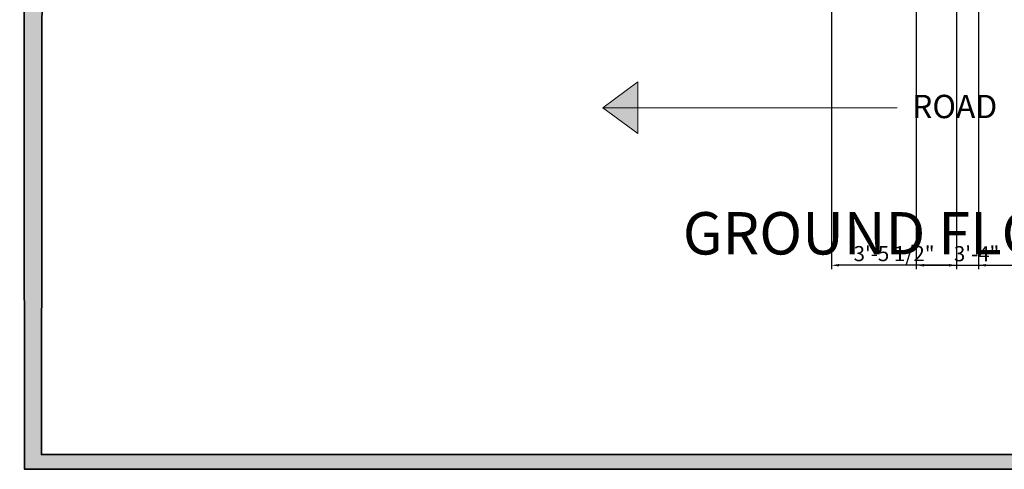
# Model space of a CAD drawing. Units: inches. Extents: x 1804 to 3296, y 909 to 2477.
# Tile 1 of 31: x 1804 to 2130, y 909 to 1059. Entities that reach past the tile are written whole.
import ezdxf

# ---------------------------------------------------------------- set-up
doc = ezdxf.new("R2010")
doc.units = ezdxf.units.IN
for name, color, linetype, lineweight in [('A-ANNO-DIMS', 2, 'Continuous', 18), ('A-ANNO-SYMB', 7, 'Continuous', 18), ('A-ANNO-TTLB', 156, 'Continuous', 35), ('A-WALL-PATT', 10, 'Continuous', 13), ('TEXT', 190, 'Continuous', 18)]:
    doc.layers.add(name, color=color, linetype=linetype, lineweight=lineweight)
doc.styles.get("Standard").update_dxf_attribs({"font": 'arial.ttf'})
doc.dimstyles.new('ISO-25', dxfattribs={"dimtxt": 5, "dimasz": 2.5, "dimexe": 1.25, "dimexo": 0.625, "dimtad": 1, "dimdec": 0, "dimlunit": 4, "dimtxsty": 'Standard', "dimcen": 2.5, "dimadec": 0, "dimazin": 0, "dimtfac": 1, "dimtdec": 0, "dimtmove": 0, "dimatfit": 3, "dimfxl": 1, "dimarcsym": 0})

# ---------------------------------------------------------------- blocks, each defined once
blk = doc.blocks.new('ROAD-DIRECTION')
h = blk.add_hatch(color=256)
h.dxf.hatch_style = 1
h.paths.add_polyline_path([(11.63, 8.56), (0, 8.56), (11.63, 0)])
h.paths.add_polyline_path([(11.63, 17.12), (0, 8.56), (11.63, 8.56)])
for p, q in [((0, 8.56), (11.63, 17.12)), ((11.63, 0), (11.63, 17.12)), ((97.65, 8.56), (0, 8.56)), ((0, 8.56), (11.63, 0))]:
    blk.add_line(p, q)
blk = doc.blocks.new('*D59')
at = {"layer": 'A-ANNO-DIMS', "color": 0, "lineweight": -2, "transparency": 16777216}
for p, q in [((2121.83, 1590.3), (2121.83, 975.89)), ((2161.83, 1590.3), (2161.83, 975.89)), ((2124.33, 977.14), (2159.33, 977.14))]:
    blk.add_line(p, q, dxfattribs=at)
at = {"layer": 'A-ANNO-DIMS', "color": 0, "lineweight": 100, "transparency": 16777216}
for points in [[(2124.33, 977.56), (2124.33, 976.72), (2121.83, 977.14)], [(2159.33, 977.56), (2159.33, 976.72), (2161.83, 977.14)]]:
    blk.add_solid(points, dxfattribs=at)
at = {"layer": 'Defpoints', "color": 0, "lineweight": 100, "transparency": 16777216}
for p in [(2121.83, 1590.92), (2161.83, 1590.92), (2161.83, 977.14)]:
    blk.add_point(p, dxfattribs=at)
at = {"layer": 'A-ANNO-DIMS', "color": 0, "transparency": 16777216, "insert": (2141.83, 980.32), "char_height": 5, "attachment_point": 5}
blk.add_mtext('3\'-4"', dxfattribs=at)
blk = doc.blocks.new('*D60')
at = {"layer": 'A-ANNO-DIMS', "color": 0, "lineweight": -2, "transparency": 16777216}
for p, q in [((2073.08, 1544.95), (2073.08, 975.89)), ((2114.58, 1543.75), (2114.58, 975.89)), ((2112.08, 977.14), (2075.58, 977.14))]:
    blk.add_line(p, q, dxfattribs=at)
at = {"layer": 'A-ANNO-DIMS', "color": 0, "lineweight": 100, "transparency": 16777216}
for points in [[(2075.58, 977.56), (2075.58, 976.72), (2073.08, 977.14)], [(2112.08, 977.56), (2112.08, 976.72), (2114.58, 977.14)]]:
    blk.add_solid(points, dxfattribs=at)
at = {"layer": 'Defpoints', "color": 0, "lineweight": 100, "transparency": 16777216}
for p in [(2073.08, 1545.58), (2114.58, 1544.38), (2073.08, 977.14)]:
    blk.add_point(p, dxfattribs=at)
at = {"layer": 'A-ANNO-DIMS', "color": 0, "transparency": 16777216, "insert": (2093.83, 980.35), "char_height": 5, "attachment_point": 5}
blk.add_mtext('3\'-5 1/2"', dxfattribs=at)
blk = doc.blocks.new('*D61')
at = {"layer": 'A-ANNO-DIMS', "color": 0, "lineweight": -2, "transparency": 16777216}
for p, q in [((2101.21, 1137.44), (2101.21, 975.89)), ((2141.21, 1137.44), (2141.21, 975.89)), ((2103.71, 977.14), (2138.71, 977.14))]:
    blk.add_line(p, q, dxfattribs=at)
at = {"layer": 'A-ANNO-DIMS', "color": 0, "lineweight": 100, "transparency": 16777216}
for points in [[(2103.71, 977.56), (2103.71, 976.72), (2101.21, 977.14)], [(2138.71, 977.56), (2138.71, 976.72), (2141.21, 977.14)]]:
    blk.add_solid(points, dxfattribs=at)
at = {"layer": 'Defpoints', "color": 0, "lineweight": 100, "transparency": 16777216}
for p in [(2101.21, 1138.07), (2141.21, 1138.07), (2141.21, 977.14)]:
    blk.add_point(p, dxfattribs=at)
at = {"layer": 'A-ANNO-DIMS', "color": 0, "transparency": 16777216, "insert": (2121.21, 980.32), "char_height": 5, "attachment_point": 5}
blk.add_mtext('3\'-4"', dxfattribs=at)

msp = doc.modelspace()

# ---------------------------------------------------------------- hatches: boundary and pattern name
at = {"layer": 'A-ANNO-TTLB'}
h = msp.add_hatch(color=256, dxfattribs=at)
h.dxf.hatch_style = 1
h.paths.add_polyline_path([(3294.53, 2476.54), (1803.79, 2476.54), (1805.43, 909.47), (3296.17, 909.47)])
h.paths.add_polyline_path([(1811, 914.33), (1812.79, 2467.54), (3285.53, 2467.54), (3283.74, 914.33)], flags=16)
h.paths.add_polyline_path([(1925.58, 1062.77), (1925.58, 1138.07), (1925.58, 1539.88), (1925.58, 1793.38), (1925.58, 1830.04), (2325.54, 1830.04), (2325.54, 1793.38), (2325.54, 1586.42), (2325.54, 1138.07), (2325.54, 1062.77)], flags=0)
h.paths.add_polyline_path([(1997.22, 1029.4), (2008.85, 1037.96), (2008.85, 1020.84)], flags=0)
h.paths.add_polyline_path([(1934.58, 1138.07), (1934.58, 1147.07), (2078.77, 1147.07), (2078.77, 1138.07), (2060.94, 1138.07)], flags=0)
h.paths.add_polyline_path([(1944.35, 1138.07), (1944.35, 1147.07), (2056.05, 1147.07), (2056.05, 1138.07)], flags=0)
h.paths.add_polyline_path([(2222.24, 1037.96), (2233.87, 1029.4), (2222.24, 1020.84)], flags=0)
h.paths.add_polyline_path([(2061.94, 1139.07), (2061.94, 1146.07), (2077.77, 1146.07), (2077.77, 1139.07)], flags=0)
h.paths.add_polyline_path([(2149.58, 1138.07), (2149.58, 1269.44), (2158.58, 1269.44), (2158.58, 1326.69), (2149.58, 1326.69), (2149.58, 1340.94), (2139.6, 1340.94), (2139.6, 1434.25), (2149.58, 1434.25), (2149.58, 1447.36), (2158.58, 1447.36), (2158.58, 1423.87), (2158.58, 1408.06), (2198.46, 1408.06), (2198.46, 1412.56), (2282.65, 1412.56), (2282.65, 1465.94), (2316.54, 1465.94), (2316.54, 1590.92), (2192.86, 1590.92), (2192.86, 1595.3), (2291.17, 1595.3), (2291.17, 1590.92), (2316.54, 1590.92), (2316.54, 1784.38), (2300.24, 1784.38), (2300.24, 1757.47), (2268, 1757.47), (2268, 1681.04), (2180.87, 1681.04), (2180.87, 1757.47), (2148.63, 1757.47), (2148.63, 1784.38), (2119.08, 1784.38), (2119.08, 1585.58), (2114.58, 1585.58), (2114.58, 1784.38), (2064.11, 1784.38), (2046.28, 1784.38), (2046.28, 1760.38), (1958.58, 1760.38), (1958.58, 1664.38), (1934.58, 1664.38), (1934.58, 1784.38), (1934.58, 1793.38), (2046.28, 1793.38), (2064.11, 1793.38), (2119.08, 1793.38), (2230.78, 1793.38), (2230.78, 1784.38), (2268, 1784.38), (2300.24, 1784.38), (2316.54, 1784.38), (2316.54, 1590.92), (2316.54, 1373.73), (2316.54, 1138.07)], flags=0)
h.paths.add_polyline_path([(2209.19, 1166.63), (2209.19, 1175.63), (2158.58, 1175.63), (2209.19, 1223.63), (2209.19, 1231.63), (2183.88, 1231.63), (2183.88, 1301.66), (2242.59, 1301.66), (2242.59, 1326.69), (2316.54, 1326.69), (2272.59, 1271.63), (2272.59, 1223.63), (2316.54, 1175.63), (2272.59, 1175.63), (2272.59, 1166.63)], flags=0)
h.paths.add_polyline_path([(1947.77, 1345.22), (1947.77, 1457.48), (1991.2, 1457.48), (1991.2, 1451.7), (1991.2, 1352.18), (1991.2, 1345.22)], flags=0)
h.paths.add_polyline_path([(2209.19, 1271.63), (2262.59, 1271.63), (2262.59, 1311.85), (2272.59, 1301.66), (2272.59, 1271.63), (2269.92, 1269.63), (2270.59, 1269.63), (2270.59, 1225.63), (2211.19, 1225.63), (2211.19, 1269.63), (2211.86, 1269.63)], flags=0)
h.paths.add_polyline_path([(2000.34, 1378.21), (2000.34, 1429.71), (2025.22, 1429.71), (2025.22, 1378.21)], flags=0)
h.paths.add_polyline_path([(2001.34, 1379.21), (2001.34, 1428.71), (2024.22, 1428.71), (2024.22, 1379.21)], flags=0)
h.paths.add_polyline_path([(2012.34, 1390.21), (2012.34, 1417.71), (2013.22, 1417.71), (2013.22, 1390.21)], flags=0)
h.paths.add_polyline_path([(2237.56, 1331.19), (2237.56, 1340.18), (2238.62, 1340.18), (2238.62, 1386.84), (2241.04, 1386.84), (2242.06, 1386.84), (2242.06, 1408.06), (2316.54, 1331.19)], flags=0)
h.paths.add_polyline_path([(1953.73, 1464.35), (1953.73, 1498.59), (1981.74, 1498.59), (1981.74, 1464.35)], flags=0)
h.paths.add_polyline_path([(1987.63, 1462.08), (1987.63, 1500.95), (2104.07, 1500.95), (2104.07, 1462.08), (2099.27, 1462.08), (1993.6, 1462.08)], flags=0)
h.paths.add_polyline_path([(1956.06, 1481.47, -1), (1979.41, 1481.47, -1)], flags=0)
edge = h.paths.add_edge_path(flags=0)
edge.add_ellipse((2299.53, 1438.37), major_axis=(0.31, 21.36), ratio=0.670333, start_angle=0, end_angle=360)
h.paths.add_polyline_path([(2297.39, 1438.37, -1), (2301.67, 1438.37, -1)], flags=0)
h.paths.add_polyline_path([(2591.54, 1163.23), (2591.54, 1179.38), (2591.54, 1379.68), (2591.54, 1395.84), (2734.5, 1395.84), (2734.5, 1379.68), (2734.5, 1179.38), (2734.5, 1163.23)], flags=0)
h.paths.add_polyline_path([(2592.54, 1164.23), (2592.54, 1166.23), (2733.5, 1166.23), (2733.5, 1164.23)], flags=0)
h.paths.add_polyline_path([(2592.54, 1180.38), (2592.54, 1378.68), (2733.5, 1378.68), (2733.5, 1180.38)], flags=0)
h.paths.add_polyline_path([(2593.54, 1181.38), (2593.54, 1377.68), (2732.5, 1377.68), (2732.5, 1181.38)], flags=0)
h.paths.add_polyline_path([(2594.54, 1182.38), (2594.54, 1376.68), (2731.5, 1376.68), (2731.5, 1182.38)], flags=0)
h.paths.add_polyline_path([(1936.95, 1697.46), (1936.95, 1736.46), (1955.41, 1736.46), (1955.41, 1697.46)], flags=0)
h.paths.add_polyline_path([(1938.48, 1718.36), (1938.48, 1734.92), (1953.65, 1734.92), (1953.65, 1718.36)], flags=0)
h.paths.add_polyline_path([(1944.75, 1726.64, -1), (1947.37, 1726.64, -1)], flags=0)
h.paths.add_polyline_path([(2592.54, 1394.84), (2733.5, 1394.84), (2733.5, 1392.84), (2592.54, 1392.84)], flags=0)
h.paths.add_polyline_path([(1976.61, 1762.5), (1976.61, 1781.44), (2012.79, 1781.44), (2012.79, 1762.5)], flags=0)
h.paths.add_polyline_path([(1979.57, 1771.97, -1), (1991.39, 1771.97, -1)], flags=0)
h.paths.add_polyline_path([(1995.36, 1771.97, -1), (2007.18, 1771.97, -1)], flags=0)
h.paths.add_polyline_path([(2251.51, 1744.53), (2268, 1730.05), (2251.51, 1730.05)], flags=0)
h.paths.add_polyline_path([(2047.28, 1785.38), (2047.28, 1792.38), (2063.11, 1792.38), (2063.11, 1785.38)], flags=0)
h.paths.add_polyline_path([(2155.08, 1770.92, -1), (2174.42, 1770.92, -1)], flags=0)
h.paths.add_polyline_path([(2188.59, 1758.27), (2188.59, 1772.81), (2222.3, 1772.81), (2222.3, 1758.27)], flags=0)
h.paths.add_polyline_path([(2223.97, 1758.27), (2223.97, 1772.81), (2257.68, 1772.81), (2257.68, 1758.27)], flags=0)
h.paths.add_polyline_path([(2274.45, 1770.92, -1), (2293.8, 1770.92, -1)], flags=0)
h.paths.add_polyline_path([(2591.54, 1582.09), (2591.54, 1782.39), (2734.5, 1782.39), (2734.5, 1582.09)], flags=0)
h.paths.add_polyline_path([(2592.54, 1583.09), (2592.54, 1781.39), (2733.5, 1781.39), (2733.5, 1583.09)], flags=0)
h.paths.add_polyline_path([(2593.54, 1584.09), (2593.54, 1780.39), (2732.5, 1780.39), (2732.5, 1584.09)], flags=0)
h.paths.add_polyline_path([(2594.54, 1585.09), (2594.54, 1779.39), (2731.5, 1779.39), (2731.5, 1585.09)], flags=0)
h.paths.add_polyline_path([(1922.17, 1978.79), (1922.17, 2295.08), (1922.17, 2296.08), (2115.67, 2296.08), (2115.67, 2384.31), (2115.67, 2385.31), (2322.12, 2385.31), (2323.12, 2385.31), (2323.12, 1979.79), (2323.12, 1978.79), (1923.17, 1978.79)], flags=0)
h.paths.add_polyline_path([(1922.17, 1978.79), (1922.17, 2051.31), (1922.17, 2214.86), (1922.17, 2296.08), (2115.67, 2296.08), (2115.67, 2385.31), (2323.12, 2385.31), (2323.12, 2280.42), (2323.12, 1978.79), (2115.67, 1978.79)], flags=0)
h.paths.add_polyline_path([(1923.17, 1979.79), (1923.17, 2050.31), (2115.67, 2050.31), (2115.67, 2051.31), (1923.17, 2051.31), (1923.17, 2213.86), (1923.17, 2214.86), (1923.17, 2295.08), (1990.02, 2295.08), (1990.02, 2214.86), (1991.02, 2214.86), (1991.02, 2295.08), (2115.67, 2295.08), (2115.67, 1979.79), (2116.67, 1979.79), (2116.67, 2304.18), (2116.67, 2384.31), (2322.12, 2384.31), (2322.12, 2280.42), (2322.12, 1979.79), (2115.67, 1979.79)], flags=0)
h.paths.add_polyline_path([(2972.46, 1192.5), (2972.46, 1196.92), (2995.47, 1196.92), (2995.47, 1255.47), (2995.09, 1255.47), (2987.42, 1249.39), (2980.08, 1255.47), (2978.05, 1255.47), (2978.05, 1257.24), (2995.47, 1257.24), (2995.47, 1261.58), (3015.37, 1261.58), (3015.37, 1333.28), (3015.37, 1414.4), (3032.82, 1414.4), (3032.82, 1333.28), (3032.82, 1261.58), (3052.66, 1261.58), (3052.66, 1255.47), (3079.86, 1255.47), (3078.72, 1254.57), (3081.47, 1252.29), (3078.56, 1249.99), (3075.81, 1252.26), (3072.57, 1249.69), (3070.36, 1251.52), (3067.67, 1249.39), (3060.34, 1255.47), (3052.66, 1255.47), (3052.66, 1196.92), (3054.58, 1196.92), (3074, 1196.92), (3074, 1192.5), (3052.66, 1192.5), (2995.47, 1192.5)], flags=0)
h.paths.add_polyline_path([(2490.75, 1979.27), (2490.75, 1980.27), (2596.87, 1980.27), (2596.87, 2051.8), (2596.87, 2052.8), (2596.87, 2216.35), (2596.87, 2297.57), (2717.32, 2297.57), (2710.57, 2305.62), (2724.07, 2305.62), (2717.32, 2297.57), (2782.37, 2297.57), (2782.37, 2395.8), (3006.82, 2395.8), (3006.82, 1981.27), (3093.73, 1981.27), (3093.73, 1980.27), (3047.51, 1980.27), (3046.37, 1979.37), (3049.11, 1977.1), (3046.2, 1974.79), (3043.46, 1977.07), (3040.21, 1974.49), (3038, 1976.32), (3035.32, 1974.2), (3027.98, 1980.27), (2871.83, 1980.27), (2871.83, 1981.27), (2791.37, 1981.27), (2791.37, 2050.8), (2597.87, 2050.8), (2597.87, 1980.27), (2597.87, 1979.27), (2546.27, 1979.27), (2545.12, 1978.37), (2547.87, 1976.1), (2544.96, 1973.79), (2542.22, 1976.07), (2538.97, 1973.49), (2536.76, 1975.32), (2534.07, 1973.2), (2526.74, 1979.27)], flags=0)
h.paths.add_polyline_path([(2597.87, 2051.8), (2606.87, 2051.8), (2606.87, 2258.39), (2597.87, 2258.39), (2597.87, 2296.57), (2606.87, 2296.57), (2606.87, 2262.39), (2782.37, 2262.39), (2782.37, 2296.57), (2790.37, 2296.57), (2790.37, 2262.39), (2791.37, 2262.39), (2791.37, 2305.67), (2791.37, 2385.8), (2996.82, 2385.8), (2996.82, 2339.85), (3006.82, 2339.85), (3006.82, 2250.12), (2997.82, 2250.12), (2997.82, 1981.27), (2996.82, 1981.27), (2872.83, 1981.27), (2872.83, 1991.8), (2871.83, 1991.8), (2871.83, 2050.8), (2790.37, 2050.8), (2597.87, 2050.8)], flags=0)
h.paths.add_polyline_path([(2179.93, 2153.92), (2179.93, 2353.97), (2259.98, 2353.97), (2259.98, 2153.92)], flags=0)
h.paths.add_polyline_path([(2180.93, 2154.92), (2180.93, 2352.97), (2258.98, 2352.97), (2258.98, 2154.92)], flags=0)
h.paths.add_polyline_path([(2960.87, 1608.49), (2960.87, 1753.62), (3070.9, 1753.62), (3070.9, 1608.49)], flags=0)
h.paths.add_polyline_path([(2961.87, 1609.49), (2961.87, 1752.62), (3069.9, 1752.62), (3069.9, 1609.49)], flags=0)
h.paths.add_polyline_path([(2962.87, 1610.49), (2962.87, 1751.62), (3068.9, 1751.62), (3068.9, 1610.49)], flags=0)
h.paths.add_polyline_path([(2963.87, 1611.49), (2963.87, 1750.62), (3067.9, 1750.62), (3067.9, 1611.49)], flags=0)
h.paths.add_polyline_path([(2782.37, 2051.8), (2782.37, 2216.32), (2791.37, 2216.32), (2791.37, 2051.8), (2872.83, 2051.8), (2872.83, 2068.56), (2884.67, 2068.56), (2884.67, 2085.33), (2896.51, 2085.33), (2896.51, 2102.09), (2908.36, 2102.09), (2908.36, 2118.85), (2920.2, 2118.85), (2920.2, 2135.62), (2932.05, 2135.62), (2932.05, 2145.3), (2925.08, 2145.3), (2925.08, 2203.2), (2996.82, 2203.2), (2996.82, 2145.3), (2953.82, 2145.3), (2872.83, 2051.8), (2790.37, 2051.8)], flags=0)
h.paths.add_polyline_path([(2717.32, 2238.65), (2710.57, 2246.7), (2724.07, 2246.7)], flags=0)
h.paths.add_polyline_path([(2003.09, 1122.79), (2017.16, 1122.79), (2017.16, 1138.74), (2003.09, 1138.74)], flags=8)
h.paths.add_polyline_path([(2174.76, 1792.72), (2188.83, 1792.72), (2188.83, 1808.66), (2174.76, 1808.66)], flags=8)
h.paths.add_polyline_path([(1987.95, 1792.51), (2002.02, 1792.51), (2002.02, 1808.45), (1987.95, 1808.45)], flags=8)
h.paths.add_polyline_path([(2148.79, 1289.26), (2160.46, 1289.26), (2160.46, 1305.2), (2148.79, 1305.2)], flags=8)
h.paths.add_polyline_path([(2115.36, 1133.57), (2127.04, 1133.57), (2127.04, 1149.51), (2115.36, 1149.51)], flags=8)
h.paths.add_polyline_path([(2237.58, 1421.48), (2249.25, 1421.48), (2249.25, 1437.43), (2237.58, 1437.43)], flags=8)
h.paths.add_polyline_path([(2134.99, 1584.32), (2146.66, 1584.32), (2146.66, 1600.26), (2134.99, 1600.26)], flags=8)
h.paths.add_polyline_path([(2101.95, 1557.31), (2113.62, 1557.31), (2113.62, 1573.25), (2101.95, 1573.25)], flags=8)
h.paths.add_polyline_path([(2937.85, 1156.77), (3120.41, 1156.77), (3120.41, 1185.72), (2937.85, 1185.72)], flags=8)
h.paths.add_polyline_path([(2980.71, 1786.71), (3050.06, 1786.71), (3050.06, 1802.66), (2980.71, 1802.66)], flags=8)
h.paths.add_polyline_path([(2869.28, 1661.96), (2938.62, 1661.96), (2938.62, 1690.8), (2869.28, 1690.8)], flags=8)
h.paths.add_polyline_path([(3092.27, 1674.86), (3161.62, 1674.86), (3161.62, 1690.8), (3092.27, 1690.8)], flags=8)
h.paths.add_polyline_path([(2980.71, 1674.86), (3050.06, 1674.86), (3050.06, 1690.8), (2980.71, 1690.8)], flags=8)
h.paths.add_polyline_path([(2649.07, 1678.23), (2674.53, 1678.23), (2674.53, 1714.76), (2649.07, 1714.76)], flags=8)
h.paths.add_polyline_path([(2530.84, 1981.63), (2549.13, 1981.63), (2549.13, 1997.57), (2530.84, 1997.57)], flags=8)
h.paths.add_polyline_path([(3031.29, 1981.77), (3049.58, 1981.77), (3049.58, 1997.71), (3031.29, 1997.71)], flags=8)
h.paths.add_polyline_path([(2715.38, 1911.9), (2851.54, 1911.9), (2851.54, 1940.85), (2715.38, 1940.85)], flags=8)
h.paths.add_polyline_path([(2015.23, 1927.36), (2205.42, 1927.36), (2205.42, 1956.3), (2015.23, 1956.3)], flags=8)
h.paths.add_polyline_path([(2671.84, 2057.84), (2702.75, 2057.84), (2702.75, 2073.79), (2671.84, 2073.79)], flags=8)
h.paths.add_polyline_path([(2678.5, 2316.52), (2765.26, 2316.52), (2765.26, 2332.46), (2678.5, 2332.46)], flags=8)
h.paths.add_polyline_path([(2678.48, 2271.96), (2736.41, 2271.96), (2736.41, 2287.9), (2678.48, 2287.9)], flags=8)
h.paths.add_polyline_path([(2019.2, 972.79), (2243.21, 972.79), (2243.21, 1001.74), (2019.2, 1001.74)], flags=8)
h.paths.add_polyline_path([(2097.06, 1021.56), (2132.16, 1021.56), (2132.16, 1037.51), (2097.06, 1037.51)], flags=8)
h.paths.add_polyline_path([(2182.47, 1360.48), (2207.35, 1360.48), (2207.35, 1376.42), (2182.47, 1376.42)], flags=8)
h.paths.add_polyline_path([(2261.12, 1361.77), (2295.01, 1361.77), (2295.01, 1377.71), (2261.12, 1377.71)], flags=8)
h.paths.add_polyline_path([(2245.75, 1511.51), (2278.44, 1511.51), (2278.44, 1527.46), (2245.75, 1527.46)], flags=8)
h.paths.add_polyline_path([(1991.16, 1296.29), (2060.51, 1296.29), (2060.51, 1312.23), (1991.16, 1312.23)], flags=8)
h.paths.add_polyline_path([(2187, 1651.35), (2246.71, 1651.35), (2246.71, 1667.29), (2187, 1667.29)], flags=8)
h.paths.add_polyline_path([(1976.49, 1684.81), (2068.63, 1684.81), (2068.63, 1700.76), (1976.49, 1700.76)], flags=8)
at = {"layer": 'A-WALL-PATT'}
h = msp.add_hatch(color=256, dxfattribs=at)
h.dxf.hatch_style = 1
h.paths.add_polyline_path([(2119.08, 1544.38), (1925.58, 1544.38), (1925.58, 1539.88), (2119.08, 1539.88)])
h.paths.add_polyline_path([(2119.08, 1545.58), (2114.58, 1545.58), (2114.58, 1544.38), (2119.08, 1544.38)])
h.paths.add_polyline_path([(1965.87, 1658.79), (1965.87, 1679.09), (1955.57, 1679.09), (1955.57, 1658.79)], flags=9)
h.paths.add_polyline_path([(2293.18, 1677.29), (2293.18, 1697.58), (2282.88, 1697.58), (2282.88, 1677.29)], flags=9)
h.paths.add_polyline_path([(2271.13, 1545.23), (2287.53, 1545.23), (2287.53, 1555.53), (2271.13, 1555.53)], flags=9)
h.paths.add_polyline_path([(2303.26, 1488.52), (2303.26, 1508.82), (2292.95, 1508.82), (2292.95, 1488.52)], flags=9)
h.paths.add_polyline_path([(2271.13, 1393.15), (2287.53, 1393.15), (2287.53, 1403.45), (2271.13, 1403.45)], flags=9)
h.paths.add_polyline_path([(2306.48, 1361.45), (2306.48, 1377.86), (2296.18, 1377.86), (2296.18, 1361.45)], flags=9)
h.paths.add_polyline_path([(2174.54, 1361.45), (2174.54, 1377.86), (2164.23, 1377.86), (2164.23, 1361.45)], flags=9)
h.paths.add_polyline_path([(1968.21, 1333.34), (1968.21, 1353.64), (1957.91, 1353.64), (1957.91, 1333.34)], flags=9)
h.paths.add_polyline_path([(2003.09, 1122.79), (2017.16, 1122.79), (2017.16, 1138.74), (2003.09, 1138.74)], flags=9)
h.paths.add_polyline_path([(2174.76, 1792.72), (2188.83, 1792.72), (2188.83, 1808.66), (2174.76, 1808.66)], flags=9)
h.paths.add_polyline_path([(1987.95, 1792.51), (2002.02, 1792.51), (2002.02, 1808.45), (1987.95, 1808.45)], flags=9)
h.paths.add_polyline_path([(2148.79, 1289.26), (2160.46, 1289.26), (2160.46, 1305.2), (2148.79, 1305.2)], flags=9)
h.paths.add_polyline_path([(2115.36, 1133.57), (2127.04, 1133.57), (2127.04, 1149.51), (2115.36, 1149.51)], flags=9)
h.paths.add_polyline_path([(2237.58, 1421.48), (2249.25, 1421.48), (2249.25, 1437.43), (2237.58, 1437.43)], flags=9)
h.paths.add_polyline_path([(2134.99, 1584.32), (2146.66, 1584.32), (2146.66, 1600.26), (2134.99, 1600.26)], flags=9)
h.paths.add_polyline_path([(2101.95, 1557.31), (2113.62, 1557.31), (2113.62, 1573.25), (2101.95, 1573.25)], flags=9)
h.paths.add_polyline_path([(2937.85, 1156.77), (3120.41, 1156.77), (3120.41, 1185.72), (2937.85, 1185.72)], flags=9)
h.paths.add_polyline_path([(2980.71, 1786.71), (3050.06, 1786.71), (3050.06, 1802.66), (2980.71, 1802.66)], flags=9)
h.paths.add_polyline_path([(2869.28, 1661.96), (2938.62, 1661.96), (2938.62, 1690.8), (2869.28, 1690.8)], flags=9)
h.paths.add_polyline_path([(3092.27, 1674.86), (3161.62, 1674.86), (3161.62, 1690.8), (3092.27, 1690.8)], flags=9)
h.paths.add_polyline_path([(2980.71, 1674.86), (3050.06, 1674.86), (3050.06, 1690.8), (2980.71, 1690.8)], flags=9)
h.paths.add_polyline_path([(2649.07, 1678.23), (2674.53, 1678.23), (2674.53, 1714.76), (2649.07, 1714.76)], flags=9)
h.paths.add_polyline_path([(2530.84, 1981.63), (2549.13, 1981.63), (2549.13, 1997.57), (2530.84, 1997.57)], flags=9)
h.paths.add_polyline_path([(3031.29, 1981.77), (3049.58, 1981.77), (3049.58, 1997.71), (3031.29, 1997.71)], flags=9)
h.paths.add_polyline_path([(2715.38, 1911.9), (2851.54, 1911.9), (2851.54, 1940.85), (2715.38, 1940.85)], flags=9)
h.paths.add_polyline_path([(2015.23, 1927.36), (2205.42, 1927.36), (2205.42, 1956.3), (2015.23, 1956.3)], flags=9)
h.paths.add_polyline_path([(2671.84, 2057.84), (2702.75, 2057.84), (2702.75, 2073.79), (2671.84, 2073.79)], flags=9)
h.paths.add_polyline_path([(2678.5, 2316.52), (2765.26, 2316.52), (2765.26, 2332.46), (2678.5, 2332.46)], flags=9)
h.paths.add_polyline_path([(2678.48, 2271.96), (2736.41, 2271.96), (2736.41, 2287.9), (2678.48, 2287.9)], flags=9)
h.paths.add_polyline_path([(2019.2, 972.79), (2243.21, 972.79), (2243.21, 1001.74), (2019.2, 1001.74)], flags=9)
h.paths.add_polyline_path([(2097.06, 1021.56), (2132.16, 1021.56), (2132.16, 1037.51), (2097.06, 1037.51)], flags=9)
h.paths.add_polyline_path([(2182.47, 1360.48), (2207.35, 1360.48), (2207.35, 1376.42), (2182.47, 1376.42)], flags=9)
h.paths.add_polyline_path([(2261.12, 1361.77), (2295.01, 1361.77), (2295.01, 1377.71), (2261.12, 1377.71)], flags=9)
h.paths.add_polyline_path([(2245.75, 1511.51), (2278.44, 1511.51), (2278.44, 1527.46), (2245.75, 1527.46)], flags=9)
h.paths.add_polyline_path([(1991.16, 1296.29), (2060.51, 1296.29), (2060.51, 1312.23), (1991.16, 1312.23)], flags=9)
h.paths.add_polyline_path([(2187, 1651.35), (2246.71, 1651.35), (2246.71, 1667.29), (2187, 1667.29)], flags=9)
h.paths.add_polyline_path([(1976.49, 1684.81), (2068.63, 1684.81), (2068.63, 1700.76), (1976.49, 1700.76)], flags=9)
h = msp.add_hatch(color=256, dxfattribs=at)
h.dxf.hatch_style = 1
h.paths.add_polyline_path([(2149.58, 1147.07), (2141.21, 1147.07), (2141.21, 1144.07), (2141.21, 1138.07), (2149.58, 1138.07)])
h.paths.add_polyline_path([(2101.21, 1144.07, -0.01877), (2101.32, 1147.07), (2078.77, 1147.07), (2078.77, 1138.07), (2101.21, 1138.07)])
h.paths.add_polyline_path([(2060.94, 1147.07), (2056.05, 1147.07), (2056.05, 1138.07), (2060.94, 1138.07)])
h.paths.add_polyline_path([(1944.35, 1147.07), (1934.58, 1147.07), (1934.58, 1138.07), (1944.35, 1138.07)])
h.paths.add_polyline_path([(2158.58, 1269.44), (2149.58, 1269.44), (2149.58, 1138.07), (2158.58, 1138.07)])
h.paths.add_polyline_path([(2003.09, 1122.79), (2017.16, 1122.79), (2017.16, 1138.74), (2003.09, 1138.74)], flags=9)
h.paths.add_polyline_path([(2174.76, 1792.72), (2188.83, 1792.72), (2188.83, 1808.66), (2174.76, 1808.66)], flags=9)
h.paths.add_polyline_path([(1987.95, 1792.51), (2002.02, 1792.51), (2002.02, 1808.45), (1987.95, 1808.45)], flags=9)
h.paths.add_polyline_path([(2148.79, 1289.26), (2160.46, 1289.26), (2160.46, 1305.2), (2148.79, 1305.2)], flags=9)
h.paths.add_polyline_path([(2115.36, 1133.57), (2127.04, 1133.57), (2127.04, 1149.51), (2115.36, 1149.51)], flags=9)
h.paths.add_polyline_path([(2237.58, 1421.48), (2249.25, 1421.48), (2249.25, 1437.43), (2237.58, 1437.43)], flags=9)
h.paths.add_polyline_path([(2134.99, 1584.32), (2146.66, 1584.32), (2146.66, 1600.26), (2134.99, 1600.26)], flags=9)
h.paths.add_polyline_path([(2101.95, 1557.31), (2113.62, 1557.31), (2113.62, 1573.25), (2101.95, 1573.25)], flags=9)
h.paths.add_polyline_path([(2937.85, 1156.77), (3120.41, 1156.77), (3120.41, 1185.72), (2937.85, 1185.72)], flags=9)
h.paths.add_polyline_path([(2980.71, 1786.71), (3050.06, 1786.71), (3050.06, 1802.66), (2980.71, 1802.66)], flags=9)
h.paths.add_polyline_path([(2869.28, 1661.96), (2938.62, 1661.96), (2938.62, 1690.8), (2869.28, 1690.8)], flags=9)
h.paths.add_polyline_path([(3092.27, 1674.86), (3161.62, 1674.86), (3161.62, 1690.8), (3092.27, 1690.8)], flags=9)
h.paths.add_polyline_path([(2980.71, 1674.86), (3050.06, 1674.86), (3050.06, 1690.8), (2980.71, 1690.8)], flags=9)
h.paths.add_polyline_path([(2649.07, 1678.23), (2674.53, 1678.23), (2674.53, 1714.76), (2649.07, 1714.76)], flags=9)
h.paths.add_polyline_path([(2530.84, 1981.63), (2549.13, 1981.63), (2549.13, 1997.57), (2530.84, 1997.57)], flags=9)
h.paths.add_polyline_path([(3031.29, 1981.77), (3049.58, 1981.77), (3049.58, 1997.71), (3031.29, 1997.71)], flags=9)
h.paths.add_polyline_path([(2715.38, 1911.9), (2851.54, 1911.9), (2851.54, 1940.85), (2715.38, 1940.85)], flags=9)
h.paths.add_polyline_path([(2015.23, 1927.36), (2205.42, 1927.36), (2205.42, 1956.3), (2015.23, 1956.3)], flags=9)
h.paths.add_polyline_path([(2671.84, 2057.84), (2702.75, 2057.84), (2702.75, 2073.79), (2671.84, 2073.79)], flags=9)
h.paths.add_polyline_path([(2678.5, 2316.52), (2765.26, 2316.52), (2765.26, 2332.46), (2678.5, 2332.46)], flags=9)
h.paths.add_polyline_path([(2678.48, 2271.96), (2736.41, 2271.96), (2736.41, 2287.9), (2678.48, 2287.9)], flags=9)
h.paths.add_polyline_path([(2019.2, 972.79), (2243.21, 972.79), (2243.21, 1001.74), (2019.2, 1001.74)], flags=9)
h.paths.add_polyline_path([(2097.06, 1021.56), (2132.16, 1021.56), (2132.16, 1037.51), (2097.06, 1037.51)], flags=9)
h.paths.add_polyline_path([(2182.47, 1360.48), (2207.35, 1360.48), (2207.35, 1376.42), (2182.47, 1376.42)], flags=9)
h.paths.add_polyline_path([(2261.12, 1361.77), (2295.01, 1361.77), (2295.01, 1377.71), (2261.12, 1377.71)], flags=9)
h.paths.add_polyline_path([(2245.75, 1511.51), (2278.44, 1511.51), (2278.44, 1527.46), (2245.75, 1527.46)], flags=9)
h.paths.add_polyline_path([(1991.16, 1296.29), (2060.51, 1296.29), (2060.51, 1312.23), (1991.16, 1312.23)], flags=9)
h.paths.add_polyline_path([(2187, 1651.35), (2246.71, 1651.35), (2246.71, 1667.29), (2187, 1667.29)], flags=9)
h.paths.add_polyline_path([(1976.49, 1684.81), (2068.63, 1684.81), (2068.63, 1700.76), (1976.49, 1700.76)], flags=9)
h = msp.add_hatch(color=256, dxfattribs=at)
h.dxf.hatch_style = 1
h.paths.add_polyline_path([(2158.58, 1275.49), (2155.29, 1275.49), (2149.58, 1275.49), (2149.58, 1269.44), (2158.58, 1269.44)])
h.paths.add_polyline_path([(2158.58, 1326.69), (2149.58, 1326.69), (2149.58, 1319.33), (2155.29, 1319.33), (2158.58, 1319.33)])
h.paths.add_polyline_path([(2158.58, 1402.2), (2158.58, 1423.87), (2158.58, 1447.36), (2149.58, 1447.36), (2149.58, 1423.87), (2149.58, 1340.94), (2149.58, 1326.69), (2158.58, 1326.69), (2158.58, 1354.23)])
h.paths.add_polyline_path([(1965.87, 1658.79), (1965.87, 1679.09), (1955.57, 1679.09), (1955.57, 1658.79)], flags=9)
h.paths.add_polyline_path([(2293.18, 1677.29), (2293.18, 1697.58), (2282.88, 1697.58), (2282.88, 1677.29)], flags=9)
h.paths.add_polyline_path([(2271.13, 1545.23), (2287.53, 1545.23), (2287.53, 1555.53), (2271.13, 1555.53)], flags=9)
h.paths.add_polyline_path([(2303.26, 1488.52), (2303.26, 1508.82), (2292.95, 1508.82), (2292.95, 1488.52)], flags=9)
h.paths.add_polyline_path([(2271.13, 1393.15), (2287.53, 1393.15), (2287.53, 1403.45), (2271.13, 1403.45)], flags=9)
h.paths.add_polyline_path([(2306.48, 1361.45), (2306.48, 1377.86), (2296.18, 1377.86), (2296.18, 1361.45)], flags=9)
h.paths.add_polyline_path([(2189.9, 1340.62), (2206.31, 1340.62), (2206.31, 1350.92), (2189.9, 1350.92)], flags=9)
h.paths.add_polyline_path([(2174.54, 1361.45), (2174.54, 1377.86), (2164.23, 1377.86), (2164.23, 1361.45)], flags=9)
h.paths.add_polyline_path([(2304.24, 1240.8), (2304.24, 1261.09), (2293.94, 1261.09), (2293.94, 1240.8)], flags=9)
h.paths.add_polyline_path([(2227.19, 1188.73), (2247.49, 1188.73), (2247.49, 1199.03), (2227.19, 1199.03)], flags=9)
h.paths.add_polyline_path([(2181.93, 1144.21), (2181.93, 1160.62), (2171.63, 1160.62), (2171.63, 1144.21)], flags=9)
h.paths.add_polyline_path([(1968.21, 1333.34), (1968.21, 1353.64), (1957.91, 1353.64), (1957.91, 1333.34)], flags=9)
h.paths.add_polyline_path([(2029.78, 1203.53), (2053.95, 1203.53), (2053.95, 1213.83), (2029.78, 1213.83)], flags=9)
h.paths.add_polyline_path([(2576.51, 1671.88), (2576.51, 1692.17), (2566.21, 1692.17), (2566.21, 1671.88)], flags=9)
h.paths.add_polyline_path([(2566.99, 1269.67), (2566.99, 1289.96), (2556.68, 1289.96), (2556.68, 1269.67)], flags=9)
h.paths.add_polyline_path([(2581.85, 1269.17), (2581.85, 1289.46), (2571.54, 1289.46), (2571.54, 1269.17)], flags=9)
h.paths.add_polyline_path([(2650.71, 1409.75), (2674.89, 1409.75), (2674.89, 1420.05), (2650.71, 1420.05)], flags=9)
h.paths.add_polyline_path([(2003.09, 1122.79), (2017.16, 1122.79), (2017.16, 1138.74), (2003.09, 1138.74)], flags=9)
h.paths.add_polyline_path([(2174.76, 1792.72), (2188.83, 1792.72), (2188.83, 1808.66), (2174.76, 1808.66)], flags=9)
h.paths.add_polyline_path([(1987.95, 1792.51), (2002.02, 1792.51), (2002.02, 1808.45), (1987.95, 1808.45)], flags=9)
h.paths.add_polyline_path([(2148.79, 1289.26), (2160.46, 1289.26), (2160.46, 1305.2), (2148.79, 1305.2)], flags=9)
h.paths.add_polyline_path([(2115.36, 1133.57), (2127.04, 1133.57), (2127.04, 1149.51), (2115.36, 1149.51)], flags=9)
h.paths.add_polyline_path([(2237.58, 1421.48), (2249.25, 1421.48), (2249.25, 1437.43), (2237.58, 1437.43)], flags=9)
h.paths.add_polyline_path([(2134.99, 1584.32), (2146.66, 1584.32), (2146.66, 1600.26), (2134.99, 1600.26)], flags=9)
h.paths.add_polyline_path([(2101.95, 1557.31), (2113.62, 1557.31), (2113.62, 1573.25), (2101.95, 1573.25)], flags=9)
h.paths.add_polyline_path([(2937.85, 1156.77), (3120.41, 1156.77), (3120.41, 1185.72), (2937.85, 1185.72)], flags=9)
h.paths.add_polyline_path([(2980.71, 1786.71), (3050.06, 1786.71), (3050.06, 1802.66), (2980.71, 1802.66)], flags=9)
h.paths.add_polyline_path([(2869.28, 1661.96), (2938.62, 1661.96), (2938.62, 1690.8), (2869.28, 1690.8)], flags=9)
h.paths.add_polyline_path([(3092.27, 1674.86), (3161.62, 1674.86), (3161.62, 1690.8), (3092.27, 1690.8)], flags=9)
h.paths.add_polyline_path([(2980.71, 1674.86), (3050.06, 1674.86), (3050.06, 1690.8), (2980.71, 1690.8)], flags=9)
h.paths.add_polyline_path([(2649.07, 1678.23), (2674.53, 1678.23), (2674.53, 1714.76), (2649.07, 1714.76)], flags=9)
h.paths.add_polyline_path([(2530.84, 1981.63), (2549.13, 1981.63), (2549.13, 1997.57), (2530.84, 1997.57)], flags=9)
h.paths.add_polyline_path([(3031.29, 1981.77), (3049.58, 1981.77), (3049.58, 1997.71), (3031.29, 1997.71)], flags=9)
h.paths.add_polyline_path([(2715.38, 1911.9), (2851.54, 1911.9), (2851.54, 1940.85), (2715.38, 1940.85)], flags=9)
h.paths.add_polyline_path([(2015.23, 1927.36), (2205.42, 1927.36), (2205.42, 1956.3), (2015.23, 1956.3)], flags=9)
h.paths.add_polyline_path([(2671.84, 2057.84), (2702.75, 2057.84), (2702.75, 2073.79), (2671.84, 2073.79)], flags=9)
h.paths.add_polyline_path([(2678.5, 2316.52), (2765.26, 2316.52), (2765.26, 2332.46), (2678.5, 2332.46)], flags=9)
h.paths.add_polyline_path([(2678.48, 2271.96), (2736.41, 2271.96), (2736.41, 2287.9), (2678.48, 2287.9)], flags=9)
h.paths.add_polyline_path([(2019.2, 972.79), (2243.21, 972.79), (2243.21, 1001.74), (2019.2, 1001.74)], flags=9)
h.paths.add_polyline_path([(2097.06, 1021.56), (2132.16, 1021.56), (2132.16, 1037.51), (2097.06, 1037.51)], flags=9)
h.paths.add_polyline_path([(2182.47, 1360.48), (2207.35, 1360.48), (2207.35, 1376.42), (2182.47, 1376.42)], flags=9)
h.paths.add_polyline_path([(2261.12, 1361.77), (2295.01, 1361.77), (2295.01, 1377.71), (2261.12, 1377.71)], flags=9)
h.paths.add_polyline_path([(2245.75, 1511.51), (2278.44, 1511.51), (2278.44, 1527.46), (2245.75, 1527.46)], flags=9)
h.paths.add_polyline_path([(1991.16, 1296.29), (2060.51, 1296.29), (2060.51, 1312.23), (1991.16, 1312.23)], flags=9)
h.paths.add_polyline_path([(2187, 1651.35), (2246.71, 1651.35), (2246.71, 1667.29), (2187, 1667.29)], flags=9)
h.paths.add_polyline_path([(1976.49, 1684.81), (2068.63, 1684.81), (2068.63, 1700.76), (1976.49, 1700.76)], flags=9)

# ---------------------------------------------------------------- linework, layer by layer
at = {"layer": 'A-ANNO-TTLB'}
for points in [[(1803.79, 2476.54), (3294.53, 2476.54), (3296.17, 909.47), (1805.43, 909.47)], [(1812.79, 2467.54), (3285.53, 2467.54), (3283.74, 914.33), (1811, 914.33)]]:
    msp.add_lwpolyline(points, close=True, dxfattribs=at)

# ---------------------------------------------------------------- block references
at = {"layer": 'A-ANNO-SYMB'}
msp.add_blockref('ROAD-DIRECTION', (1997.22, 1020.84), dxfattribs=at)

# ---------------------------------------------------------------- texts
at = {"layer": 'TEXT', "attachment_point": 1}
for s, width, gutter_width, insert, char_height in [('ROAD', 163.3261, 38.69, (2099.84, 1033.66), 7.737), ('GROUND FLOOR PLAN', 296.512, 70.23, (2023.76, 994.76), 14.0468)]:
    msp.add_mtext_dynamic_manual_height_columns(s, width=width, gutter_width=gutter_width, heights=[0], dxfattribs=dict(at, insert=insert, char_height=char_height))

# ---------------------------------------------------------------- dimensions: what is measured, and where the dimension line sits
at = {"layer": 'A-ANNO-DIMS'}
for base, p1, p2, picture, middle in [((2161.83, 977.14), (2121.83, 1590.92), (2161.83, 1590.92), '*D59', (2141.83, 980.32)), ((2073.08, 977.14), (2114.58, 1544.38), (2073.08, 1545.58), '*D60', (2093.83, 980.35)), ((2141.21, 977.14), (2101.21, 1138.07), (2141.21, 1138.07), '*D61', (2121.21, 980.32))]:
    dim = msp.add_linear_dim(base=base, p1=p1, p2=p2, dimstyle='ISO-25', override={"dimdec": 1, "dimlfac": 1, "dimrnd": 0, "dimzin": 1, "dimdsep": 46, "dimlunit": 4, "dimfrac": 2}, dxfattribs=at)
    dim.commit()
    dim.dimension.update_dxf_attribs({"geometry": picture, "text_midpoint": middle})

doc.saveas('drawing.dxf')
